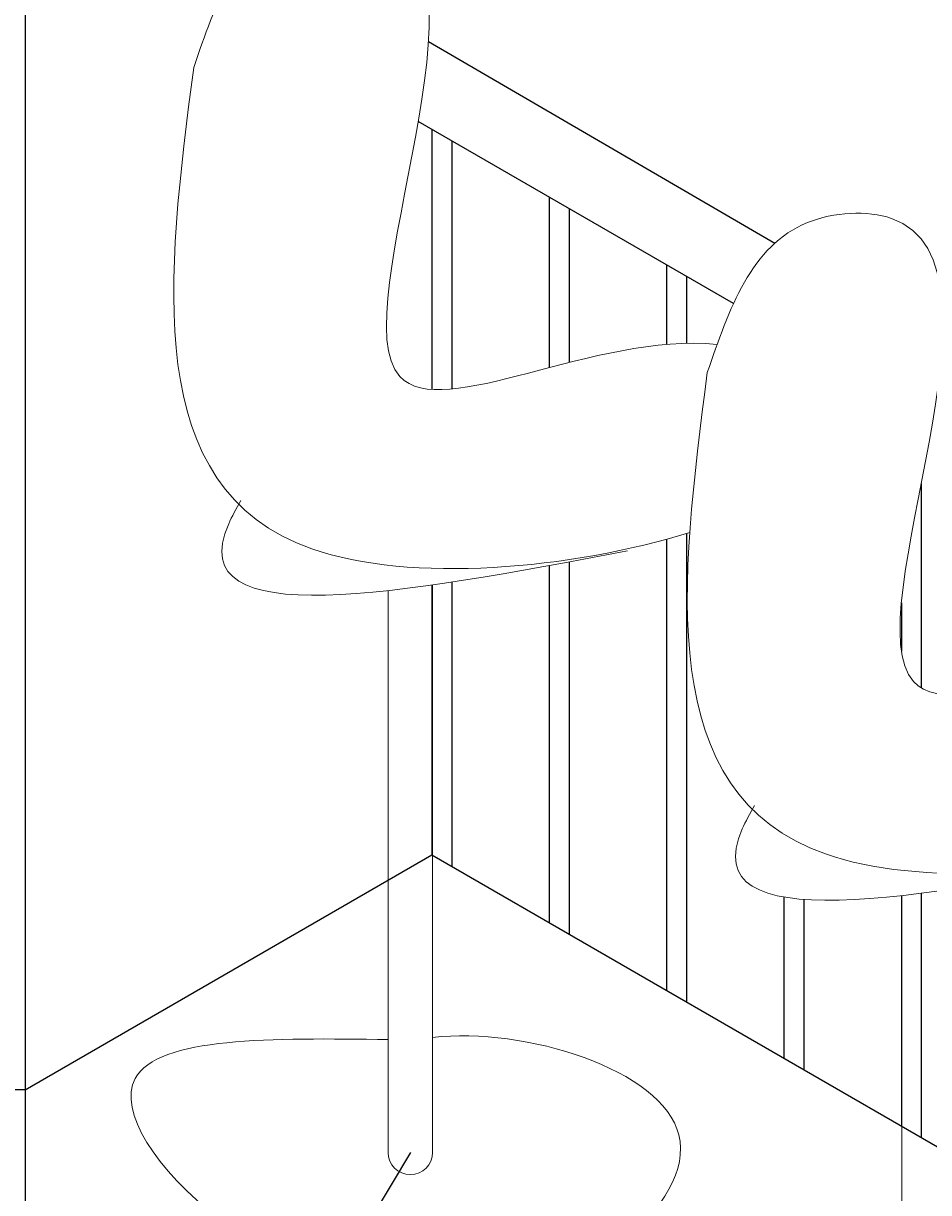
# Model space of a CAD drawing. Units: metres. Extents: x -2391 to 4922, y -635 to 4845.
# Tile 4 of 37: x -2049 to -1367, y 528 to 1408. Entities that reach past the tile are written whole.
import ezdxf

# ---------------------------------------------------------------- set-up
doc = ezdxf.new("R2010")
doc.units = ezdxf.units.M
doc.header["$MEASUREMENT"] = 0
for name, color, linetype, lineweight in [('A-ANNO-DIMS', 2, 'Continuous', 18), ('A-FLOR-FIXT', 3, 'Continuous', 25), ('A-FURN', 8, 'Continuous', 18)]:
    doc.layers.add(name, color=color, linetype=linetype, lineweight=lineweight)
doc.styles.get("Standard").update_dxf_attribs({"font": 'arial.ttf'})
doc.dimstyles.get("Standard").update_dxf_attribs({"dimtxt": 5, "dimasz": 4, "dimexe": 0.18, "dimexo": 0.0625, "dimgap": 0.09, "dimtad": 0, "dimtih": 1, "dimtoh": 1, "dimdec": 0, "dimzin": 0, "dimdsep": 46, "dimtxsty": 'Standard', "dimcen": 0.09, "dimadec": 0, "dimazin": 0, "dimtfac": 1, "dimtdec": 0, "dimtofl": 0, "dimtmove": 0, "dimatfit": 3, "dimfxl": 1, "dimtolj": 1, "dimtzin": 0, "dimarcsym": 0})

# ---------------------------------------------------------------- blocks, each defined once
blk = doc.blocks.new('STOOL-BAR')
blk.add_line((193.66, 114.21), (193.66, 537.32))
for points, knots in [([(47.24, 931.27), (26.82, 772.78), (-15.55, 443.76), (639.86, 614.21), (403.75, 766.18), (59.87, 548.32), (308.37, 1061.03), (87.86, 1049.28), (63.7, 979.1), (47.24, 931.27)], [0, 0, 0, 0, 373.373325, 775.091582, 839.205201, 1103.589215, 1452.822506, 1516.235646, 1651.960559, 1651.960559, 1651.960559, 1651.960559]), ([(82.71, 605.1), (79.37, 599.07), (25.39, 501.43), (205.15, 535.32), (373.81, 567.12)], [0, 0, 0, 0, 19.816883, 320.720948, 320.720948, 320.720948, 320.720948])]:
    blk.add_open_spline(points, degree=3, knots=knots)
blk = doc.blocks.new('*D8')
at = {"layer": 'A-ANNO-DIMS', "color": 0, "lineweight": -2, "transparency": 16777216}
for p, q in [((-2047.33, 3005.21), (-2047.33, -631.4)), ((4577.76, 2350.21), (4577.76, -631.4)), ((-2043.33, -631.22), (1257.62, -631.22)), ((4573.76, -631.22), (1272.8, -631.22))]:
    blk.add_line(p, q, dxfattribs=at)
at = {"layer": 'A-ANNO-DIMS', "color": 0, "transparency": 16777216}
for points in [[(-2043.33, -630.56), (-2043.33, -631.89), (-2047.33, -631.22)], [(4573.76, -630.56), (4573.76, -631.89), (4577.76, -631.22)]]:
    blk.add_solid(points, dxfattribs=at)
at = {"layer": 'Defpoints', "color": 0, "transparency": 16777216}
for p in [(-2047.33, 3005.28), (4577.76, 2350.28), (4577.76, -631.22)]:
    blk.add_point(p, dxfattribs=at)
at = {"layer": 'A-ANNO-DIMS', "color": 0, "transparency": 16777216, "insert": (1265.21, -631.22), "char_height": 5, "attachment_point": 5}
blk.add_mtext('\\A1;6625', dxfattribs=at)
blk = doc.blocks.new('*D10')
at = {"layer": 'A-ANNO-DIMS', "color": 0, "lineweight": -2, "transparency": 16777216}
for p, q in [((550.68, 4505.28), (-2384.01, 4505.28)), ((-2383.83, 4501.28), (-2383.83, 2107.92)), ((-2383.83, -290.72), (-2383.83, 2102.63)), ((-488.55, -294.72), (-2384.01, -294.72))]:
    blk.add_line(p, q, dxfattribs=at)
at = {"layer": 'A-ANNO-DIMS', "color": 0, "transparency": 16777216}
for points in [[(-2384.5, 4501.28), (-2383.17, 4501.28), (-2383.83, 4505.28)], [(-2384.5, -290.72), (-2383.17, -290.72), (-2383.83, -294.72)]]:
    blk.add_solid(points, dxfattribs=at)
at = {"layer": 'Defpoints', "color": 0, "transparency": 16777216}
for p in [(-2383.83, 4505.28), (550.74, 4505.28), (-488.49, -294.72)]:
    blk.add_point(p, dxfattribs=at)
at = {"layer": 'A-ANNO-DIMS', "color": 0, "transparency": 16777216, "insert": (-2383.83, 2105.28), "char_height": 5, "attachment_point": 5}
blk.add_mtext('\\A1;4800', dxfattribs=at)
blk = doc.blocks.new('*D44')
at = {"layer": 'A-ANNO-DIMS', "color": 0, "lineweight": -2, "transparency": 16777216}
for p, q in [((-2047.4, 1505.28), (-2384.01, 1505.28)), ((-2383.83, 1501.28), (-2383.83, 1057.92)), ((-2383.83, 609.28), (-2383.83, 1052.63)), ((-2047.4, 605.28), (-2384.01, 605.28))]:
    blk.add_line(p, q, dxfattribs=at)
at = {"layer": 'A-ANNO-DIMS', "color": 0, "transparency": 16777216}
for points in [[(-2384.5, 1501.28), (-2383.17, 1501.28), (-2383.83, 1505.28)], [(-2384.5, 609.28), (-2383.17, 609.28), (-2383.83, 605.28)]]:
    blk.add_solid(points, dxfattribs=at)
at = {"layer": 'Defpoints', "color": 0, "transparency": 16777216}
for p in [(-2047.33, 1505.28), (-2383.83, 605.28), (-2047.33, 605.28)]:
    blk.add_point(p, dxfattribs=at)
at = {"layer": 'A-ANNO-DIMS', "color": 0, "transparency": 16777216, "insert": (-2383.83, 1055.28), "char_height": 5, "attachment_point": 5}
blk.add_mtext('\\A1;900', dxfattribs=at)
blk = doc.blocks.new('*D46')
at = {"layer": 'A-ANNO-DIMS', "color": 0, "lineweight": -2, "transparency": 16777216}
for p, q in [((-2047.3, 1505.33), (-1887.13, 1801.4)), ((-1883.7, 1799.34), (-1087.36, 1368.5)), ((-281.24, 932.38), (-1077.58, 1363.21)), ((-437.81, 634.57), (-277.64, 930.64))]:
    blk.add_line(p, q, dxfattribs=at)
at = {"layer": 'A-ANNO-DIMS', "color": 0, "transparency": 16777216}
for points in [[(-1883.38, 1799.92), (-1884.01, 1798.75), (-1887.21, 1801.24)], [(-280.92, 932.97), (-281.56, 931.8), (-277.72, 930.48)]]:
    blk.add_solid(points, dxfattribs=at)
at = {"layer": 'Defpoints', "color": 0, "transparency": 16777216}
for p in [(-2047.33, 1505.28), (-277.72, 930.48), (-437.84, 634.52)]:
    blk.add_point(p, dxfattribs=at)
at = {"layer": 'A-ANNO-DIMS', "color": 0, "transparency": 16777216, "insert": (-1082.47, 1365.86), "char_height": 5, "attachment_point": 5}
blk.add_mtext('\\A1;1830', dxfattribs=at)
blk = doc.blocks.new('*D50')
at = {"layer": 'A-ANNO-DIMS', "color": 0, "lineweight": -2, "transparency": 16777216}
for p, q in [((-1757.26, 558), (-1929.17, 268.59)), ((-1370.51, 328.28), (-1542.41, 38.86)), ((-1925.64, 266.7), (-1740.15, 156.52)), ((-1545.76, 41.06), (-1731.25, 151.24))]:
    blk.add_line(p, q, dxfattribs=at)
at = {"layer": 'A-ANNO-DIMS', "color": 0, "transparency": 16777216}
for points in [[(-1925.3, 267.28), (-1925.98, 266.13), (-1929.08, 268.75)], [(-1545.42, 41.63), (-1546.1, 40.49), (-1542.32, 39.02)]]:
    blk.add_solid(points, dxfattribs=at)
at = {"layer": 'Defpoints', "color": 0, "transparency": 16777216}
for p in [(-1757.23, 558.06), (-1370.48, 328.33), (-1929.08, 268.75)]:
    blk.add_point(p, dxfattribs=at)
at = {"layer": 'A-ANNO-DIMS', "color": 0, "transparency": 16777216, "insert": (-1735.7, 153.88), "char_height": 5, "attachment_point": 5}
blk.add_mtext('\\A1;449.8', dxfattribs=at)

msp = doc.modelspace()

# ---------------------------------------------------------------- linework, layer by layer
at = {"layer": 'A-FLOR-FIXT'}
for p, q in [((-2047.3343, 1505.2763), (-2047.3343, 605.2763)), ((-1743.5797, 1394.6663), (-1482.7469, 1242.8199)), ((-1513.8865, 1197.29), (-1751.2544, 1334.3345)), ((-1741.1171, 1328.4817), (-1741.1171, 1132.5811)), ((-1726.1091, 1319.8168), (-1726.1091, 1132.9022)), ((-1652.7157, 1277.4431), (-1652.7157, 1149.0408)), ((-1637.7076, 1268.7782), (-1637.7076, 1152.9063)), ((-1564.3142, 1226.4045), (-1564.3142, 1166.5162)), ((-1549.3061, 1217.7396), (-1549.3061, 1167.3288)), ((-1372.5032, 1061.7043), (-1372.5032, 907.8381)), ((-1549.3061, 1024.1763), (-1549.3061, 671.3287)), ((-1564.3142, 1019.8041), (-1564.3142, 679.9936)), ((-1652.7157, 999.986), (-1652.7157, 731.0322)), ((-1637.7076, 1002.7429), (-1637.7076, 722.3673)), ((-1726.1091, 987.53), (-1726.1091, 773.4059)), ((-1741.1171, 985.3229), (-1741.1171, 782.0708)), ((-1387.5113, 971.8846), (-1387.5113, 935.4282)), ((-2047.3343, 605.2763), (-1741.1171, 782.0708)), ((-1741.1171, 782.0708), (-488.4886, 58.8654)), ((-1475.9128, 750.3477), (-1475.9128, 628.955)), ((-1460.9047, 748.5364), (-1460.9047, 620.2901)), ((-1387.5113, 751.3995), (-1387.5113, 577.9164)), ((-1372.5032, 753.1661), (-1372.5032, 569.2515))]:
    msp.add_line(p, q, dxfattribs=at)
at = {"layer": 'A-FURN'}
for p, q in [((-1773.9741, 558.0561), (-1773.9741, 981.1586)), ((-1740.4832, 985.4128), (-1740.4832, 558.0561))]:
    msp.add_line(p, q, dxfattribs=at)
msp.add_arc((-1757.2287, 558.0561), 16.7454, 180, 0, dxfattribs=at)
for points, knots in [([(-1526.2689, 1166.4698), (-1618.3807, 1175.9307), (-1899.5699, 1009.0778), (-1659.2657, 1504.8781), (-1879.7796, 1493.1197), (-1903.9345, 1422.9415), (-1920.3976, 1375.1107)], [588.24960444, 588.24960444, 588.24960444, 588.24960444, 753.51326986, 991.96424045, 1035.26173009, 1127.93255518, 1127.93255518, 1127.93255518, 1127.93255518]), ([(-1920.3976, 1375.1107), (-1940.811, 1216.619), (-1972.8006, 968.247), (-1635.6776, 997.0844), (-1546.8427, 1024.9417)], [0, 0, 0, 0, 254.9334036, 399.50564635, 399.50564635, 399.50564635, 399.50564635]), ([(-1884.9285, 1048.9467), (-1888.2639, 1042.9137), (-1942.2443, 945.2742), (-1762.4833, 979.1667), (-1593.8295, 1010.9651)], [0, 0, 0, 0, 19.81688277, 320.72094765, 320.72094765, 320.72094765, 320.72094765]), ([(-1773.9741, 642.9857), (-1860.7418, 644.1794), (-2081.5157, 647.2169), (-1752.1913, 347.944), (-1459.2678, 587.3777), (-1671.1165, 652.6299), (-1740.4832, 644.6157)], [0, 0, 0, 0, 131.59689154, 334.83830103, 476.92925131, 613.0889369, 613.0889369, 613.0889369, 613.0889369])]:
    msp.add_open_spline(points, degree=3, knots=knots, dxfattribs=at)

# ---------------------------------------------------------------- block references
msp.add_blockref('STOOL-BAR', (-1580.882, 214.116), dxfattribs=at)

# ---------------------------------------------------------------- dimensions: what is measured, and where the dimension line sits
at = {"layer": 'A-ANNO-DIMS'}
for base, p1, p2, angle, override, picture, middle in [((-2383.8343, 4505.2763), (-488.4886, -294.7237), (550.7419, 4505.2763), 90, {"dimdec": 0, "dimlfac": 1, "dimrnd": 0, "dimzin": 0, "dimdsep": 46, "dimlunit": 2}, '*D10', (-2383.8343, 2105.2763)), ((-277.7211, 930.4802), (-2047.3343, 1505.2763), (-437.841, 634.5176), 331.5859855, {"dimdec": 0, "dimlfac": 1, "dimrnd": 0, "dimzin": 0, "dimdsep": 46, "dimlunit": 2}, '*D46', (-1082.4677, 1365.8595)), ((-2383.8343, 605.2763), (-2047.3343, 1505.2763), (-2047.3343, 605.2763), 90, {"dimdec": 0, "dimlfac": 1, "dimrnd": 0, "dimzin": 0, "dimdsep": 46, "dimlunit": 2}, '*D44', (-2383.8343, 1055.2763)), ((-1929.0761, 268.7454), (-1370.4753, 328.3288), (-1757.2287, 558.0561), 149.2901447, {"dimdec": 1, "dimlfac": 1, "dimrnd": 0, "dimzin": 0, "dimdsep": 46, "dimlunit": 2}, '*D50', (-1735.6994, 153.8817))]:
    dim = msp.add_linear_dim(base=base, p1=p1, p2=p2, angle=angle, dimstyle='Standard', override=override, dxfattribs=at)
    dim.commit()
    dim.dimension.update_dxf_attribs({"geometry": picture, "text_midpoint": middle})
dim = msp.add_linear_dim(base=(4577.76, -631.2237), p1=(-2047.3343, 3005.2763), p2=(4577.76, 2350.2763), dimstyle='Standard', override={"dimdec": 0, "dimlfac": 1, "dimrnd": 0, "dimzin": 0, "dimdsep": 46, "dimlunit": 2}, dxfattribs=at)
dim.commit()
dim.dimension.update_dxf_attribs({"geometry": '*D8', "text_midpoint": (1265.2128, -631.2237)})

doc.saveas('drawing.dxf')
